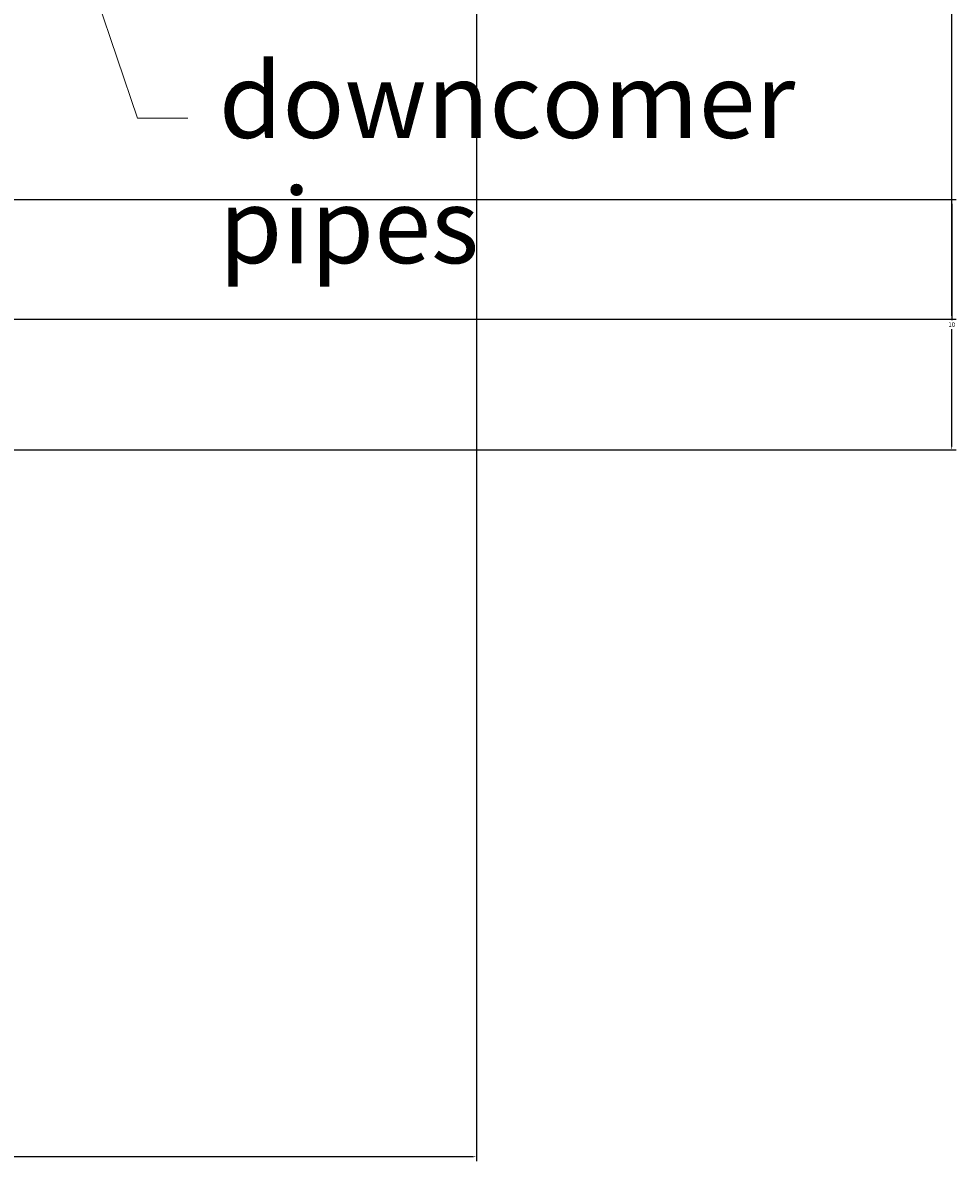
# Model space of a CAD drawing. Units: inches. Extents: x -1 to 292, y -3 to 199.
# Tile 37 of 52: x 255 to 292, y -3 to 43. Entities that reach past the tile are written whole.
import ezdxf

# ---------------------------------------------------------------- set-up
doc = ezdxf.new("R2010")
doc.units = ezdxf.units.IN
doc.header["$MEASUREMENT"] = 0
for name, color, linetype, lineweight in [('M-ANNO-LEAD', 2, 'Continuous', 18), ('M-ANNO-TEXT', 3, 'Continuous', 25), ('M-DIMS', 2, 'Continuous', 18)]:
    doc.layers.add(name, color=color, linetype=linetype, lineweight=lineweight)
doc.styles.get("Standard").update_dxf_attribs({"font": 'arial.ttf'})
doc.dimstyles.get("Standard").update_dxf_attribs({"dimtxt": 0.18, "dimasz": 0.18, "dimexe": 0.18, "dimexo": 0.0625, "dimgap": 0.09, "dimtad": 0, "dimtih": 1, "dimtoh": 1, "dimdec": 4, "dimzin": 0, "dimdsep": 46, "dimtxsty": 'Standard', "dimcen": 0.09, "dimadec": 0, "dimazin": 0, "dimtfac": 1, "dimtdec": 4, "dimtofl": 0, "dimtmove": 0, "dimatfit": 3, "dimfxl": 1, "dimtolj": 1, "dimtzin": 0, "dimarcsym": 0})

# ---------------------------------------------------------------- blocks, each defined once
blk = doc.blocks.new('*D11')
at = {"layer": 'Defpoints', "color": 0, "transparency": 16777216}
for p in [(79.013, 35.514), (292.04, 35.514), (79.013, 25.514)]:
    blk.add_point(p, dxfattribs=at)
at = {"layer": 'M-DIMS', "color": 0, "lineweight": -2, "transparency": 16777216}
for p, q in [((79.076, 35.514), (292.22, 35.514)), ((292.04, 35.334), (292.04, 30.696)), ((292.04, 25.694), (292.04, 30.332)), ((79.076, 25.514), (292.22, 25.514))]:
    blk.add_line(p, q, dxfattribs=at)
at = {"layer": 'M-DIMS', "color": 0, "transparency": 16777216}
for points in [[(292.01, 35.334), (292.07, 35.334), (292.04, 35.514)], [(292.01, 25.694), (292.07, 25.694), (292.04, 25.514)]]:
    blk.add_solid(points, dxfattribs=at)
at = {"layer": 'M-DIMS', "color": 0, "transparency": 16777216, "insert": (292.04, 30.514), "char_height": 0.18, "attachment_point": 5}
blk.add_mtext('\\A1;10', dxfattribs=at)
blk = doc.blocks.new('*D25')
at = {"layer": 'Defpoints', "color": 0, "transparency": 16777216}
for p in [(273.066, 88.419), (215.241, 88.13), (273.066, -2.71)]:
    blk.add_point(p, dxfattribs=at)
at = {"layer": 'M-DIMS', "color": 0, "lineweight": -2, "transparency": 16777216}
for p, q in [((273.066, 88.357), (273.066, -2.89)), ((215.241, 88.068), (215.241, -2.89)), ((215.421, -2.71), (243.76, -2.71)), ((272.886, -2.71), (244.547, -2.71))]:
    blk.add_line(p, q, dxfattribs=at)
at = {"layer": 'M-DIMS', "color": 0, "transparency": 16777216}
for points in [[(215.421, -2.68), (215.421, -2.74), (215.241, -2.71)], [(272.886, -2.68), (272.886, -2.74), (273.066, -2.71)]]:
    blk.add_solid(points, dxfattribs=at)
at = {"layer": 'M-DIMS', "color": 0, "transparency": 16777216, "insert": (244.153, -2.71), "char_height": 0.18, "attachment_point": 5}
blk.add_mtext('\\A1;57.83', dxfattribs=at)
blk = doc.blocks.new('*D33')
at = {"layer": 'Defpoints', "color": 0, "transparency": 16777216}
for p in [(242.955, 125.727), (292.04, 125.727), (237.933, 30.73)]:
    blk.add_point(p, dxfattribs=at)
at = {"layer": 'M-DIMS', "color": 0, "lineweight": -2, "transparency": 16777216}
for p, q in [((243.018, 125.727), (292.22, 125.727)), ((292.04, 125.547), (292.04, 78.41)), ((292.04, 30.91), (292.04, 78.046)), ((237.996, 30.73), (292.22, 30.73))]:
    blk.add_line(p, q, dxfattribs=at)
at = {"layer": 'M-DIMS', "color": 0, "transparency": 16777216}
for points in [[(292.01, 125.547), (292.07, 125.547), (292.04, 125.727)], [(292.01, 30.91), (292.07, 30.91), (292.04, 30.73)]]:
    blk.add_solid(points, dxfattribs=at)
at = {"layer": 'M-DIMS', "color": 0, "transparency": 16777216, "insert": (292.04, 78.228), "char_height": 0.18, "attachment_point": 5}
blk.add_mtext('\\A1;95', dxfattribs=at)

msp = doc.modelspace()

# ---------------------------------------------------------------- linework, layer by layer
at = {"layer": 'M-ANNO-LEAD'}
for p, q in [((255.3414, 51.2013), (259.5359, 38.7603)), ((259.5359, 38.7603), (261.5471, 38.7603))]:
    msp.add_line(p, q, dxfattribs=at)

# ---------------------------------------------------------------- texts
at = {"layer": 'M-ANNO-TEXT', "insert": (262.7836, 40.9677), "char_height": 3, "attachment_point": 1}
msp.add_mtext_dynamic_manual_height_columns('downcomer pipes', width=23.906137, gutter_width=1, heights=[0], dxfattribs=at)

# ---------------------------------------------------------------- dimensions: what is measured, and where the dimension line sits
at = {"layer": 'M-DIMS'}
for base, p1, p2, picture, middle in [((292.0399, 125.7269), (237.9333, 30.7296), (242.9552, 125.7269), '*D33', (292.0399, 78.2282)), ((292.0399, 35.5141), (79.013, 25.5141), (79.013, 35.5141), '*D11', (292.0399, 30.5141))]:
    dim = msp.add_linear_dim(base=base, p1=p1, p2=p2, angle=90, dimstyle='Standard', override={"dimdec": 0, "dimlfac": 1, "dimrnd": 0, "dimzin": 0, "dimdsep": 46, "dimlunit": 2}, dxfattribs=at)
    dim.commit()
    dim.dimension.update_dxf_attribs({"geometry": picture, "text_midpoint": middle})
dim = msp.add_linear_dim(base=(273.0659, -2.7104), p1=(215.2407, 88.1304), p2=(273.0659, 88.4191), dimstyle='Standard', override={"dimdec": 2, "dimlfac": 1, "dimrnd": 0, "dimzin": 0, "dimdsep": 46, "dimlunit": 2}, dxfattribs=at)
dim.commit()
dim.dimension.update_dxf_attribs({"geometry": '*D25', "text_midpoint": (244.1533, -2.7104)})

doc.saveas('drawing.dxf')
